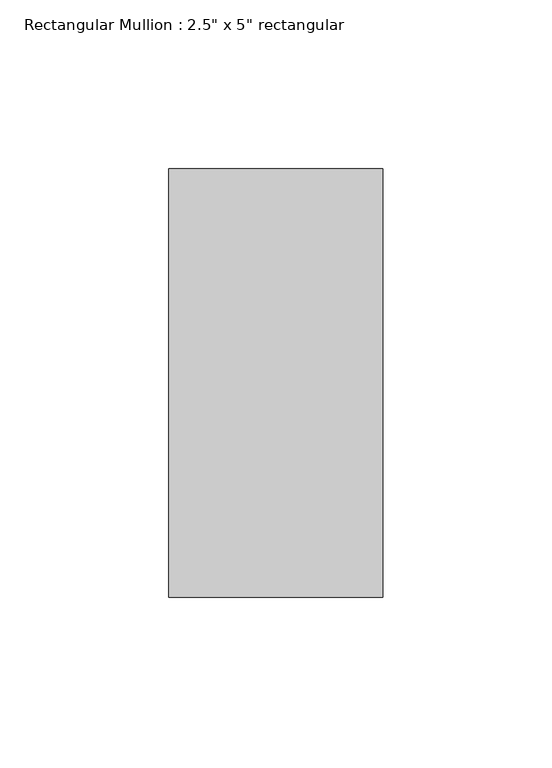
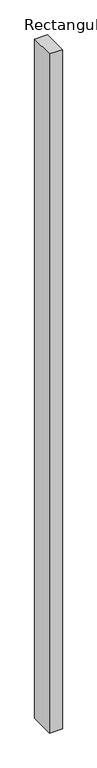
"""IFC4 building model written with IfcOpenShell, lengths in millimetres: member geometry."""

from ifc_helpers import new_model, si_unit, frame, origin, place, context, project, spatial, polyline, outline, extrude, source, transform, mapped, element, save


def member_901dee17(model_context):
    return source(origin(), model_context, "Body", "SweptSolid", [
        extrude(outline(polyline([(0.0, 63.5), (0.0, -63.5), (-63.5, -63.5), (-63.5, 63.5), (0.0, 63.5)])), frame((0.0, 0.0, -3552.5016467), z_axis=(0.0, 0.0, 1.0), x_axis=(1.0, 0.0, 0.0)), (0.0, 0.0, 1.0), 3552.5016467),
    ])


if __name__ == "__main__":
    model = new_model("IFC4")
    model_context = context("Model", 3, world=origin())
    ifc_project = project(units=[si_unit("LENGTHUNIT", "METRE", prefix="MILLI")], contexts=[model_context])
    site = spatial("IfcSite", under=ifc_project)
    building = spatial("IfcBuilding", under=site)
    placement = place(None, origin())
    member_shape = member_901dee17(model_context)
    element("IfcMember", 1, ObjectType="Rectangular Mullion : 2.5\" x 5\" rectangular", at=placement, inside=building, context=model_context, shape_type="MappedRepresentation", body=[
        mapped(member_shape, transform((0.0, 0.0, 0.0), x_axis=(1.0, 0.0, 0.0), y_axis=(0.0, 1.0, 0.0), z_axis=(0.0, 0.0, 1.0))),
    ])
    save(model, "model.ifc")

# Revit data of these elements
# Type "Rectangular Mullion : 2.5\" x 5\" rectangular"
#   built-in parameter 1007304 = 0.416667 (stored number, unit not read)
#   built-in parameter 1007301 = 0.104167 (stored number, unit not read)
#   built-in parameter 1007300 = 0.104167 (stored number, unit not read)
# Element 1 (IfcMember, "Rectangular Mullion : 2.5\" x 5\" rectangular")
#   Materials on its faces: "Aluminum"
# Materials
#   "Aluminum": class "Metal", colour RGB 247 247 247, transparency 0, Description = "Aluminum 6061", Cost = 0
